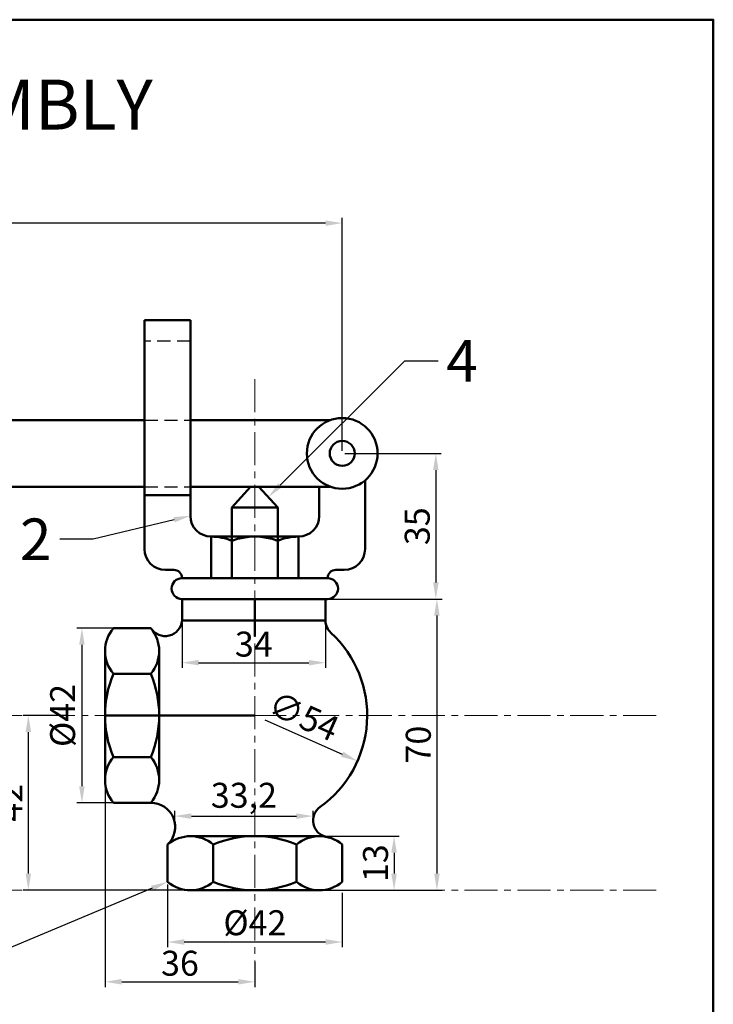
# Model space of a CAD drawing. Units: millimetres. Extents: x -25 to 763, y -62 to 306.
# Tile 7 of 7: x 597 to 763, y 69 to 306. Entities that reach past the tile are written whole.
import ezdxf
from ezdxf import colors
from ezdxf.entities.mleader import LeaderData, LeaderLine
from ezdxf.math import Vec2, Vec3

# ---------------------------------------------------------------- set-up
doc = ezdxf.new("R2010")
doc.units = ezdxf.units.MM
doc.header["$LTSCALE"] = 0.5
doc.linetypes.add('CENTER', pattern=[50.8, 31.75, -6.35, 6.35, -6.35])
doc.linetypes.add('DASHED', pattern=[19.05, 12.7, -6.35])
for name, color, linetype, lineweight in [('M-CNTR', 1, 'CENTER', 18), ('M-DIMS', 2, 'Continuous', 25), ('M-HIDN', 4, 'DASHED', 25), ('M-OUTL', 7, 'Continuous', 50), ('M-TEXT', 3, 'Continuous', 25), ('M-TTLB', 7, 'Continuous', 50)]:
    doc.layers.add(name, color=color, linetype=linetype, lineweight=lineweight)
doc.styles.get("Standard").update_dxf_attribs({"font": 'arial.ttf'})
doc.dimstyles.new('ISO-25', dxfattribs={"dimtxt": 6, "dimasz": 4, "dimexe": 1.25, "dimexo": 0.625, "dimtad": 1, "dimtoh": 1, "dimdec": 1, "dimtxsty": 'Standard', "dimcen": 2.5, "dimadec": 0, "dimazin": 0, "dimtfac": 1, "dimtdec": 1, "dimtmove": 0, "dimatfit": 3, "dimfxl": 1, "dimarcsym": 0})

# ---------------------------------------------------------------- blocks, each defined once
blk = doc.blocks.new('*D67')
at = {"layer": 'Defpoints', "color": 0, "ltscale": 0.5, "transparency": 16777216}
for p in [(382.09, 256.83), (674.09, 201.48), (382.09, 197.48)]:
    blk.add_point(p, dxfattribs=at)
at = {"layer": 'M-DIMS', "color": 0, "lineweight": -2, "ltscale": 0.5, "transparency": 16777216}
for p, q in [((382.09, 198.1), (382.09, 258.08)), ((674.09, 202.1), (674.09, 258.08)), ((670.09, 256.83), (386.09, 256.83))]:
    blk.add_line(p, q, dxfattribs=at)
at = {"layer": 'M-DIMS', "color": 0, "ltscale": 0.5, "transparency": 16777216}
for points in [[(386.09, 257.5), (386.09, 256.17), (382.09, 256.83)], [(670.09, 257.5), (670.09, 256.17), (674.09, 256.83)]]:
    blk.add_solid(points, dxfattribs=at)
at = {"layer": 'M-DIMS', "color": 0, "ltscale": 0.5, "transparency": 16777216, "insert": (528.09, 260.52), "char_height": 6, "attachment_point": 5}
blk.add_mtext('292', dxfattribs=at)
blk = doc.blocks.new('*D70')
at = {"layer": 'Defpoints', "color": 0, "ltscale": 0.5, "transparency": 16777216}
for p in [(674.09, 201.48), (665.78, 166.48), (696.6, 166.48)]:
    blk.add_point(p, dxfattribs=at)
at = {"layer": 'M-DIMS', "color": 0, "lineweight": -2, "ltscale": 0.5, "transparency": 16777216}
for p, q in [((674.72, 201.48), (697.85, 201.48)), ((696.6, 197.48), (696.6, 170.48)), ((666.4, 166.48), (697.85, 166.48))]:
    blk.add_line(p, q, dxfattribs=at)
at = {"layer": 'M-DIMS', "color": 0, "ltscale": 0.5, "transparency": 16777216}
for points in [[(695.93, 197.48), (697.26, 197.48), (696.6, 201.48)], [(695.93, 170.48), (697.26, 170.48), (696.6, 166.48)]]:
    blk.add_solid(points, dxfattribs=at)
at = {"layer": 'M-DIMS', "color": 0, "ltscale": 0.5, "transparency": 16777216, "insert": (692.9, 183.98), "char_height": 6, "attachment_point": 5, "rotation": 90}
blk.add_mtext('35', dxfattribs=at)
blk = doc.blocks.new('*D71')
at = {"layer": 'Defpoints', "color": 0, "ltscale": 0.5, "transparency": 16777216}
for p in [(665.78, 166.48), (655.35, 96.48), (696.85, 96.48)]:
    blk.add_point(p, dxfattribs=at)
at = {"layer": 'M-DIMS', "color": 0, "lineweight": -2, "ltscale": 0.5, "transparency": 16777216}
for p, q in [((666.4, 166.48), (698.1, 166.48)), ((696.85, 162.48), (696.85, 100.48)), ((655.97, 96.48), (698.1, 96.48))]:
    blk.add_line(p, q, dxfattribs=at)
at = {"layer": 'M-DIMS', "color": 0, "ltscale": 0.5, "transparency": 16777216}
for points in [[(696.19, 162.48), (697.52, 162.48), (696.85, 166.48)], [(696.19, 100.48), (697.52, 100.48), (696.85, 96.48)]]:
    blk.add_solid(points, dxfattribs=at)
at = {"layer": 'M-DIMS', "color": 0, "ltscale": 0.5, "transparency": 16777216, "insert": (693.16, 131.48), "char_height": 6, "attachment_point": 5, "rotation": 90}
blk.add_mtext('70', dxfattribs=at)
blk = doc.blocks.new('*D72')
at = {"layer": 'Defpoints', "color": 0, "ltscale": 0.5, "transparency": 16777216}
for p in [(659.79, 109.48), (659.79, 96.48), (686.56, 96.48)]:
    blk.add_point(p, dxfattribs=at)
at = {"layer": 'M-DIMS', "color": 0, "lineweight": -2, "ltscale": 0.5, "transparency": 16777216}
for p, q in [((660.41, 109.48), (687.81, 109.48)), ((686.56, 105.48), (686.56, 100.48)), ((660.41, 96.48), (687.81, 96.48))]:
    blk.add_line(p, q, dxfattribs=at)
at = {"layer": 'M-DIMS', "color": 0, "ltscale": 0.5, "transparency": 16777216}
for points in [[(685.89, 105.48), (687.22, 105.48), (686.56, 109.48)], [(685.89, 100.48), (687.22, 100.48), (686.56, 96.48)]]:
    blk.add_solid(points, dxfattribs=at)
at = {"layer": 'M-DIMS', "color": 0, "ltscale": 0.5, "transparency": 16777216, "insert": (682.87, 102.98), "char_height": 6, "attachment_point": 5, "rotation": 90}
blk.add_mtext('13', dxfattribs=at)
blk = doc.blocks.new('*D73')
at = {"layer": 'Defpoints', "color": 0, "ltscale": 0.5, "transparency": 16777216}
for p in [(632.11, 98.48), (674.11, 96.48), (674.11, 84.03)]:
    blk.add_point(p, dxfattribs=at)
at = {"layer": 'M-DIMS', "color": 0, "lineweight": -2, "ltscale": 0.5, "transparency": 16777216}
for p, q in [((632.11, 97.85), (632.11, 82.78)), ((674.11, 95.85), (674.11, 82.78)), ((636.11, 84.03), (670.11, 84.03))]:
    blk.add_line(p, q, dxfattribs=at)
at = {"layer": 'M-DIMS', "color": 0, "ltscale": 0.5, "transparency": 16777216}
for points in [[(636.11, 84.69), (636.11, 83.36), (632.11, 84.03)], [(670.11, 84.69), (670.11, 83.36), (674.11, 84.03)]]:
    blk.add_solid(points, dxfattribs=at)
at = {"layer": 'M-DIMS', "color": 0, "ltscale": 0.5, "transparency": 16777216, "insert": (653.11, 87.88), "char_height": 6, "attachment_point": 5}
blk.add_mtext('%%C42', dxfattribs=at)
blk = doc.blocks.new('*D74')
at = {"layer": 'Defpoints', "color": 0, "ltscale": 0.5, "transparency": 16777216}
for p in [(617.09, 138.46), (653.09, 79.86), (653.09, 74.46)]:
    blk.add_point(p, dxfattribs=at)
at = {"layer": 'M-DIMS', "color": 0, "lineweight": -2, "ltscale": 0.5, "transparency": 16777216}
for p, q in [((617.09, 137.83), (617.09, 73.21)), ((653.09, 79.24), (653.09, 73.21)), ((621.09, 74.46), (649.09, 74.46))]:
    blk.add_line(p, q, dxfattribs=at)
at = {"layer": 'M-DIMS', "color": 0, "ltscale": 0.5, "transparency": 16777216}
for points in [[(621.09, 75.13), (621.09, 73.79), (617.09, 74.46)], [(649.09, 75.13), (649.09, 73.79), (653.09, 74.46)]]:
    blk.add_solid(points, dxfattribs=at)
at = {"layer": 'M-DIMS', "color": 0, "ltscale": 0.5, "transparency": 16777216, "insert": (635.09, 78.15), "char_height": 6, "attachment_point": 5}
blk.add_mtext('36', dxfattribs=at)
blk = doc.blocks.new('*D75')
at = {"layer": 'Defpoints', "color": 0, "ltscale": 0.5, "transparency": 16777216}
for p in [(667.08, 114.29), (633.84, 112.69), (667.08, 113.17)]:
    blk.add_point(p, dxfattribs=at)
at = {"layer": 'M-DIMS', "color": 0, "lineweight": -2, "ltscale": 0.5, "transparency": 16777216}
for p, q in [((633.84, 113.32), (633.84, 115.54)), ((637.84, 114.29), (663.08, 114.29)), ((667.08, 113.8), (667.08, 115.54))]:
    blk.add_line(p, q, dxfattribs=at)
at = {"layer": 'M-DIMS', "color": 0, "ltscale": 0.5, "transparency": 16777216}
for points in [[(637.84, 114.96), (637.84, 113.62), (633.84, 114.29)], [(663.08, 114.96), (663.08, 113.62), (667.08, 114.29)]]:
    blk.add_solid(points, dxfattribs=at)
at = {"layer": 'M-DIMS', "color": 0, "ltscale": 0.5, "transparency": 16777216, "insert": (650.46, 118.52), "char_height": 6, "attachment_point": 5}
blk.add_mtext('33,2', dxfattribs=at)
blk = doc.blocks.new('*D76')
at = {"layer": 'Defpoints', "color": 0, "ltscale": 0.5, "transparency": 16777216}
for p in [(635.59, 161.28), (670.09, 161.28), (670.09, 151.17)]:
    blk.add_point(p, dxfattribs=at)
at = {"layer": 'M-DIMS', "color": 0, "lineweight": -2, "ltscale": 0.5, "transparency": 16777216}
for p, q in [((635.59, 160.66), (635.59, 149.92)), ((670.09, 160.66), (670.09, 149.92)), ((639.59, 151.17), (666.09, 151.17))]:
    blk.add_line(p, q, dxfattribs=at)
at = {"layer": 'M-DIMS', "color": 0, "ltscale": 0.5, "transparency": 16777216}
for points in [[(639.59, 151.84), (639.59, 150.51), (635.59, 151.17)], [(666.09, 151.84), (666.09, 150.51), (670.09, 151.17)]]:
    blk.add_solid(points, dxfattribs=at)
at = {"layer": 'M-DIMS', "color": 0, "ltscale": 0.5, "transparency": 16777216, "insert": (652.84, 154.86), "char_height": 6, "width": 15.6262, "attachment_point": 5}
blk.add_mtext('34', dxfattribs=at)
blk = doc.blocks.new('*D77')
at = {"layer": 'Defpoints', "color": 0, "ltscale": 0.5, "transparency": 16777216}
for p in [(628.41, 149.43), (677.77, 127.53)]:
    blk.add_point(p, dxfattribs=at)
at = {"layer": 'M-DIMS', "color": 0, "lineweight": -2, "ltscale": 0.5, "transparency": 16777216}
blk.add_line((655.51, 137.4), (674.11, 129.15), dxfattribs=at)
at = {"layer": 'M-DIMS', "color": 0, "ltscale": 0.5, "transparency": 16777216}
blk.add_solid([(674.38, 129.76), (673.84, 128.54), (677.77, 127.53)], dxfattribs=at)
at = {"layer": 'M-DIMS', "color": 0, "ltscale": 0.5, "transparency": 16777216, "insert": (664.55, 137.61), "char_height": 6, "attachment_point": 5, "rotation": 336.072}
blk.add_mtext('∅54', dxfattribs=at)
blk = doc.blocks.new('*D78')
at = {"layer": 'Defpoints', "color": 0, "ltscale": 0.5, "transparency": 16777216}
for p in [(598.66, 138.48), (608.6, 138.48), (653.09, 96.48)]:
    blk.add_point(p, dxfattribs=at)
at = {"layer": 'M-DIMS', "color": 0, "lineweight": -2, "ltscale": 0.5, "transparency": 16777216}
for p, q in [((607.98, 138.48), (597.41, 138.48)), ((598.66, 100.48), (598.66, 134.48)), ((652.47, 96.48), (597.41, 96.48))]:
    blk.add_line(p, q, dxfattribs=at)
at = {"layer": 'M-DIMS', "color": 0, "ltscale": 0.5, "transparency": 16777216}
for points in [[(597.99, 134.48), (599.32, 134.48), (598.66, 138.48)], [(597.99, 100.48), (599.32, 100.48), (598.66, 96.48)]]:
    blk.add_solid(points, dxfattribs=at)
at = {"layer": 'M-DIMS', "color": 0, "ltscale": 0.5, "transparency": 16777216, "insert": (595.02, 117.48), "char_height": 6, "attachment_point": 5, "rotation": 90}
blk.add_mtext('42', dxfattribs=at)
blk = doc.blocks.new('*D79')
at = {"layer": 'Defpoints', "color": 0, "ltscale": 0.5, "transparency": 16777216}
for p in [(623.59, 159.48), (611.53, 117.48), (623.59, 117.48)]:
    blk.add_point(p, dxfattribs=at)
at = {"layer": 'M-DIMS', "color": 0, "lineweight": -2, "ltscale": 0.5, "transparency": 16777216}
for p, q in [((622.97, 159.48), (610.28, 159.48)), ((611.53, 155.48), (611.53, 121.48)), ((622.97, 117.48), (610.28, 117.48))]:
    blk.add_line(p, q, dxfattribs=at)
at = {"layer": 'M-DIMS', "color": 0, "ltscale": 0.5, "transparency": 16777216}
for points in [[(610.86, 155.48), (612.19, 155.48), (611.53, 159.48)], [(610.86, 121.48), (612.19, 121.48), (611.53, 117.48)]]:
    blk.add_solid(points, dxfattribs=at)
at = {"layer": 'M-DIMS', "color": 0, "ltscale": 0.5, "transparency": 16777216, "insert": (607.67, 138.48), "char_height": 6, "attachment_point": 5, "rotation": 90}
blk.add_mtext('%%C42', dxfattribs=at)

msp = doc.modelspace()

# ---------------------------------------------------------------- linework, layer by layer
at = {"layer": 'M-CNTR', "ltscale": 0.5}
for p, q in [((653.09, 219.32), (653.09, 78.01)), ((749.56, 138.48), (561.14, 138.48)), ((749.56, 96.48), (561.14, 96.48))]:
    msp.add_line(p, q, dxfattribs=at)
at = {"layer": 'M-HIDN', "ltscale": 0.5}
for p, q in [((637.59, 228.48), (626.59, 228.48)), ((626.59, 209.48), (638.09, 209.48)), ((626.59, 193.48), (637.59, 193.48))]:
    msp.add_line(p, q, dxfattribs=at)
at = {"layer": 'M-OUTL', "ltscale": 0.5}
for p, q in [((637.59, 233.48), (626.59, 233.48)), ((626.59, 233.48), (626.59, 191.48)), ((637.59, 233.48), (637.59, 186.48)), ((492.09, 209.48), (626.59, 209.48)), ((637.59, 209.48), (671.22, 209.48)), ((679.59, 195), (679.59, 178.48)), ((626.59, 193.48), (382.09, 193.48)), ((671.22, 193.48), (637.59, 193.48)), ((647.59, 188.48), (652.09, 193.48)), ((653.09, 193.48), (652.09, 193.48)), ((653.09, 193.48), (654.09, 193.48)), ((658.59, 188.48), (654.09, 193.48)), ((668.59, 193.48), (668.59, 186.48)), ((626.59, 191.48), (637.59, 191.48)), ((626.59, 191.48), (626.59, 178.48)), ((647.59, 188.48), (647.59, 171.48)), ((658.59, 188.48), (647.59, 188.48)), ((658.59, 188.48), (658.59, 171.48)), ((642.59, 181.48), (663.59, 181.48)), ((642.59, 181.48), (642.59, 171.48)), ((658.59, 181.48), (647.59, 181.48)), ((663.59, 181.48), (663.59, 171.48)), ((633.59, 173.48), (631.59, 173.48)), ((672.59, 173.48), (674.59, 173.48)), ((635.59, 171.48), (670.59, 171.48)), ((639.37, 171.48), (635.59, 171.48)), ((635.59, 171.48), (635.59, 171.48)), ((670.59, 171.48), (670.59, 171.48)), ((635.59, 166.48), (670.59, 166.48)), ((635.59, 166.48), (635.59, 161.28)), ((670.09, 166.48), (636.09, 166.48)), ((653.09, 166.48), (653.09, 157.48)), ((670.09, 166.48), (670.09, 163.48)), ((670.09, 163.48), (670.09, 161.28)), ((635.59, 161.28), (670.09, 161.28)), ((628.09, 159.48), (619.09, 159.48)), ((617.09, 153.98), (617.09, 122.94)), ((630.09, 122.94), (630.09, 153.98)), ((628.09, 148.48), (619.09, 148.48)), ((653.09, 138.48), (617.09, 138.48)), ((619.09, 128.48), (628.09, 128.48)), ((619.09, 117.48), (628.09, 117.48)), ((668.61, 109.48), (637.57, 109.48)), ((632.11, 107.48), (632.11, 98.48)), ((643.11, 107.48), (643.11, 98.48)), ((663.11, 98.48), (663.11, 107.48)), ((674.11, 98.48), (674.11, 107.48)), ((637.57, 96.48), (668.61, 96.48))]:
    msp.add_line(p, q, dxfattribs=at)
for radius in [8.5, 8.5, 3, 3]:
    msp.add_circle((674.09, 201.48), radius, dxfattribs=at)
for centre, radius, start, end in [((642.59, 186.48), 5, 180, 270), ((663.59, 186.48), 5, 270, 0), ((642.51, 168.07), 13.41, 67.7284, 89.6517), ((653.09, 165.85), 15.62, 69.3903, 110.6097), ((663.67, 168.07), 13.41, 90.3483, 112.2716), ((631.59, 178.48), 5, 180, 270), ((674.59, 178.48), 5, 270, 0), ((633.59, 171.48), 2, 360, 90), ((672.59, 171.48), 2, 90, 180), ((635.59, 168.98), 2.5, 90, 270), ((670.59, 168.98), 2.5, 270, 90), ((631.54, 161.64), 4.07, 212.0557, 354.9864), ((674.09, 161.28), 4, 180, 227.3577), ((625.65, 153.98), 8.56, 140.0338, 219.9662), ((621.53, 153.98), 8.56, 320.0338, 39.9662), ((653.09, 138.48), 27, 305.4737, 47.3577), ((643.09, 138.48), 26, 157.3801, 202.6199), ((604.09, 138.48), 26, 337.3801, 22.6199), ((625.65, 122.98), 8.56, 140.0324, 219.9676), ((621.53, 122.98), 8.56, 320.0324, 39.9676), ((628.14, 111.69), 5.79, 313.2653, 90.5055), ((671.08, 113.23), 4, 125.4737, 258.646), ((637.61, 100.91), 8.56, 50.0324, 129.9676), ((653.11, 83.48), 26, 67.3801, 112.6199), ((668.61, 100.91), 8.56, 50.0338, 129.9662), ((637.61, 105.04), 8.56, 230.0324, 309.9676), ((653.11, 122.48), 26, 247.3801, 292.6199), ((668.61, 105.04), 8.56, 230.0338, 309.9662)]:
    msp.add_arc(centre, radius, start, end, dxfattribs=at)
at = {"layer": 'M-TTLB', "ltscale": 0.5}
msp.add_lwpolyline([(229.22, 305.74), (763.29, 305.74), (763.29, -62.45), (229.22, -62.45)], close=True, dxfattribs=at)

# ---------------------------------------------------------------- texts
at = {"layer": 'M-TTLB', "ltscale": 0.5, "insert": (403.69, 291.33), "char_height": 12, "attachment_point": 1}
msp.add_mtext_dynamic_manual_height_columns('\\pxqc;SAFETY VALVE ASSEMBLY', width=257.4414, gutter_width=12.5, heights=[0], dxfattribs=at)

# ---------------------------------------------------------------- dimensions: what is measured, and where the dimension line sits
at = {"layer": 'M-DIMS', "ltscale": 0.5}
for base, p1, p2, picture, middle in [((382.09, 256.83), (674.09, 201.48), (382.09, 197.48), '*D67', (528.09, 260.52)), ((653.09, 74.46), (617.09, 138.46), (653.09, 79.86), '*D74', (635.09, 78.15)), ((667.08, 114.29), (633.84, 112.69), (667.08, 113.17), '*D75', (650.46, 118.52))]:
    dim = msp.add_linear_dim(base=base, p1=p1, p2=p2, dimstyle='ISO-25', override={"dimclrd": 0, "dimclre": 0, "dimclrt": 0}, dxfattribs=at)
    dim.commit()
    dim.dimension.update_dxf_attribs({"geometry": picture, "text_midpoint": middle})
for base, p1, p2, picture, middle in [((696.6, 166.48), (674.09, 201.48), (665.78, 166.48), '*D70', (692.9, 183.98)), ((696.85, 96.48), (665.78, 166.48), (655.35, 96.48), '*D71', (693.16, 131.48)), ((598.66, 138.48), (653.09, 96.48), (608.6, 138.48), '*D78', (595.02, 117.48)), ((686.56, 96.48), (659.79, 109.48), (659.79, 96.48), '*D72', (682.87, 102.98))]:
    dim = msp.add_linear_dim(base=base, p1=p1, p2=p2, angle=90, dimstyle='ISO-25', override={"dimclrd": 0, "dimclre": 0, "dimclrt": 0}, dxfattribs=at)
    dim.commit()
    dim.dimension.update_dxf_attribs({"geometry": picture, "text_midpoint": middle})
for base, p1, p2, text, picture, middle in [((670.09, 151.17), (635.59, 161.28), (670.09, 161.28), '34', '*D76', (652.84, 154.86)), ((674.11, 84.03), (632.11, 98.48), (674.11, 96.48), '%%C<>', '*D73', (653.11, 87.88))]:
    dim = msp.add_linear_dim(base=base, p1=p1, p2=p2, text=text, dimstyle='ISO-25', override={"dimclrd": 0, "dimclre": 0, "dimclrt": 0}, dxfattribs=at)
    dim.commit()
    dim.dimension.update_dxf_attribs({"geometry": picture, "text_midpoint": middle})
dim = msp.add_linear_dim(base=(611.53, 117.48), p1=(623.59, 159.48), p2=(623.59, 117.48), angle=90, text='%%C<>', dimstyle='ISO-25', override={"dimclrd": 0, "dimclre": 0, "dimclrt": 0}, dxfattribs=at)
dim.commit()
dim.dimension.update_dxf_attribs({"geometry": '*D79', "text_midpoint": (607.67, 138.48)})
dim = msp.add_diameter_dim_2p(p1=(628.41, 149.43), p2=(677.77, 127.53), dimstyle='ISO-25', override={"dimclrd": 0, "dimclre": 0, "dimclrt": 0}, dxfattribs=at)
dim.commit()
dim.dimension.update_dxf_attribs({"geometry": '*D77', "text_midpoint": (662.99, 134.09), "dimtype": 163})

# ---------------------------------------------------------------- leaders
at = {"layer": 'M-TEXT', "ltscale": 0.5}
ml = msp.add_multileader_mtext('Standard', dxfattribs=at)
ml.set_content('4', color=256)
ml.set_leader_properties()
ml.build(insert=Vec2(0, 0))
ctx = ml.context
ctx.base_point, ctx.char_height, ctx.plane_origin = Vec3(697.12, 223.75), 10, Vec3(656.34, 190.98)
notes = []
notes.append((ctx, [(0, (1, 1, 0), (689.12, 223.75), (1, 0), 8, [(0, [(656.34, 190.98)], 0, [])])]))
ctx.mtext.insert, ctx.mtext.flow_direction = Vec3(699.12, 228.75), 5
ml = msp.add_multileader_mtext('Standard', dxfattribs=at)
ml.set_content('2', color=256)
ml.set_leader_properties()
ml.build(insert=Vec2(0, 0))
ctx = ml.context
ctx.base_point, ctx.char_height, ctx.plane_origin = Vec3(595.57, 180.83), 10, Vec3(637.59, 186.48)
ctx.text_align_type = 2
notes.append((ctx, [(0, (1, 1, 0), (614.2, 180.83), (-1, 0), 8, [(0, [(637.59, 186.48)], 0, [])])]))
ctx.mtext.insert, ctx.mtext.alignment, ctx.mtext.flow_direction = Vec3(604.2, 185.83), 3, 5
ml = msp.add_multileader_mtext('Standard', dxfattribs=at)
ml.set_content('1', color=256)
ml.set_leader_properties()
ml.build(insert=Vec2(0, 0))
ctx = ml.context
ctx.base_point, ctx.char_height, ctx.plane_origin = Vec3(577.79, 82.32), 10, Vec3(632.11, 98.48)
ctx.text_align_type = 2
notes.append((ctx, [(0, (1, 1, 0), (593.48, 82.32), (-1, 0), 8, [(0, [(632.11, 98.48)], 0, [])])]))
ctx.mtext.insert, ctx.mtext.alignment, ctx.mtext.flow_direction = Vec3(583.48, 87.32), 3, 5
for ctx, leaders in notes:
    for number, flags, end, landing, length, lines in leaders:
        leader = LeaderData()
        leader.index, (leader.has_last_leader_line, leader.has_dogleg_vector, leader.attachment_direction) = number, flags
        leader.last_leader_point, leader.dogleg_vector, leader.dogleg_length = Vec3(end), Vec3(landing), length
        for number, points, colour, breaks in lines:
            line = LeaderLine()
            line.index, line.vertices, line.color, line.breaks = number, Vec3.list(points), colors.encode_raw_color(colour), breaks
            leader.lines.append(line)
        ctx.leaders.append(leader)

doc.saveas('drawing.dxf')
